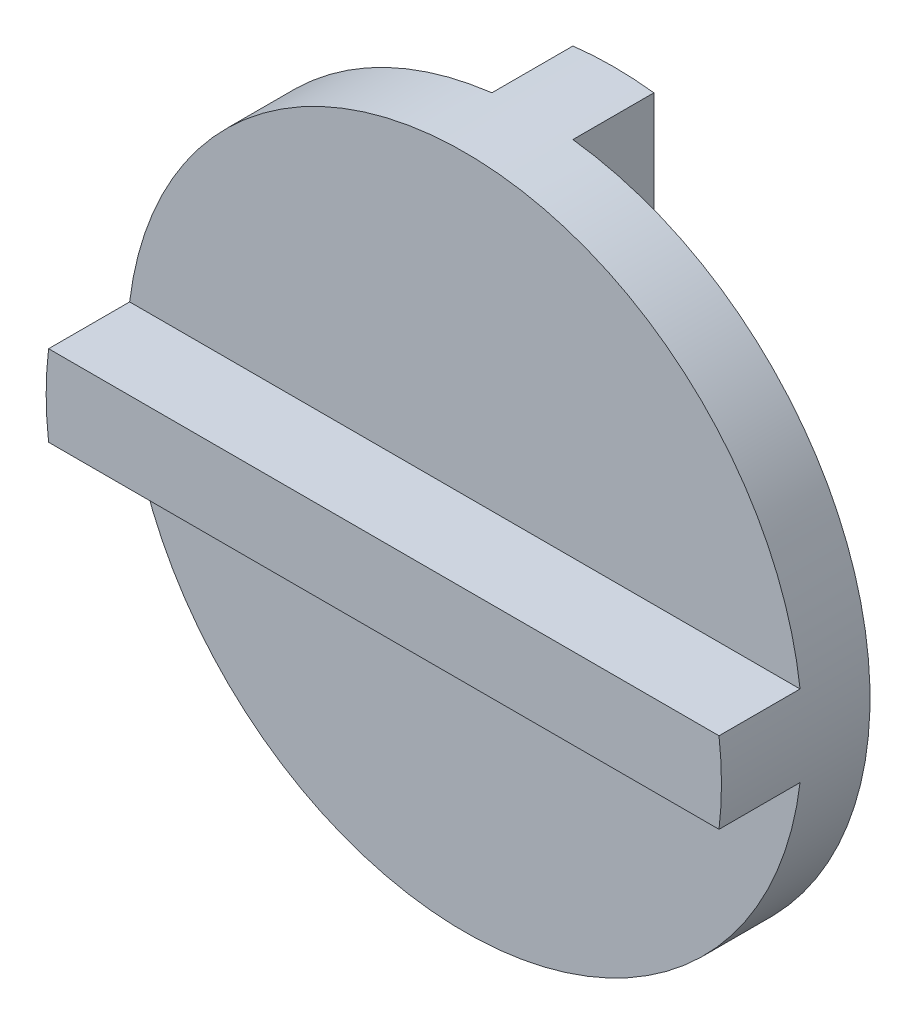
ISO-10303-21;
HEADER;
FILE_DESCRIPTION(('STEP AP214'),'2;1');
FILE_NAME('part.step','',(''),(''),'','','');
FILE_SCHEMA(('AUTOMOTIVE_DESIGN { 1 0 10303 214 1 1 1 1 }'));
ENDSEC;
DATA;
#1=APPLICATION_CONTEXT('core data for automotive mechanical design processes');
#2=APPLICATION_PROTOCOL_DEFINITION('international standard','automotive_design',2000,#1);
#3=PRODUCT_CONTEXT('',#1,'mechanical');
#4=PRODUCT('Part','Part','',(#3));
#5=PRODUCT_RELATED_PRODUCT_CATEGORY('part','',(#4));
#6=PRODUCT_DEFINITION_FORMATION('','',#4);
#7=PRODUCT_DEFINITION_CONTEXT('part definition',#1,'design');
#8=PRODUCT_DEFINITION('design','',#6,#7);
#9=PRODUCT_DEFINITION_SHAPE('','',#8);
#10=(LENGTH_UNIT() NAMED_UNIT(*) SI_UNIT(.MILLI.,.METRE.));
#11=(NAMED_UNIT(*) PLANE_ANGLE_UNIT() SI_UNIT($,.RADIAN.));
#12=(NAMED_UNIT(*) SI_UNIT($,.STERADIAN.) SOLID_ANGLE_UNIT());
#13=UNCERTAINTY_MEASURE_WITH_UNIT(LENGTH_MEASURE(1.E-05),#10,'distance_accuracy_value','');
#14=(GEOMETRIC_REPRESENTATION_CONTEXT(3) GLOBAL_UNCERTAINTY_ASSIGNED_CONTEXT((#13)) GLOBAL_UNIT_ASSIGNED_CONTEXT((#10,
#11,#12)) REPRESENTATION_CONTEXT('',''));
#15=CARTESIAN_POINT('',(0.,0.,0.));
#16=DIRECTION('',(0.,0.,1.));
#17=DIRECTION('',(1.,0.,0.));
#18=AXIS2_PLACEMENT_3D('',#15,#16,#17);
#19=CARTESIAN_POINT('',(0.,0.,-5.));
#20=DIRECTION('',(0.,0.,1.));
#21=DIRECTION('',(1.,0.,0.));
#22=AXIS2_PLACEMENT_3D('',#19,#20,#21);
#23=PLANE('',#22);
#24=DIRECTION('',(0.,1.,0.));
#25=VECTOR('',#24,1.);
#26=CARTESIAN_POINT('',(-6.,-49.6386945839634,-5.));
#27=LINE('',#26,#25);
#28=CARTESIAN_POINT('',(-6.,-49.6386945839634,-5.));
#29=VERTEX_POINT('',#28);
#30=CARTESIAN_POINT('',(-6.,49.6386945839634,-5.));
#31=VERTEX_POINT('',#30);
#32=EDGE_CURVE('E53',#29,#31,#27,.T.);
#33=ORIENTED_EDGE('',*,*,#32,.F.);
#34=CARTESIAN_POINT('',(0.,0.,-5.));
#35=DIRECTION('',(0.,0.,1.));
#36=DIRECTION('',(1.,0.,0.));
#37=AXIS2_PLACEMENT_3D('',#34,#35,#36);
#38=CIRCLE('',#37,50.);
#39=EDGE_CURVE('E60',#31,#29,#38,.T.);
#40=ORIENTED_EDGE('',*,*,#39,.F.);
#41=EDGE_LOOP('',(#33,#40));
#42=FACE_BOUND('',#41,.T.);
#43=ADVANCED_FACE('F39',(#42),#23,.F.);
#44=DIRECTION('',(0.,-1.,0.));
#45=VECTOR('',#44,1.);
#46=CARTESIAN_POINT('',(6.,-49.6386945839634,-5.));
#47=LINE('',#46,#45);
#48=CARTESIAN_POINT('',(6.,49.6386945839634,-5.));
#49=VERTEX_POINT('',#48);
#50=CARTESIAN_POINT('',(6.,-49.6386945839634,-5.));
#51=VERTEX_POINT('',#50);
#52=EDGE_CURVE('E280',#49,#51,#47,.T.);
#53=ORIENTED_EDGE('',*,*,#52,.F.);
#54=EDGE_CURVE('E43',#51,#49,#38,.T.);
#55=ORIENTED_EDGE('',*,*,#54,.F.);
#56=EDGE_LOOP('',(#53,#55));
#57=FACE_BOUND('',#56,.T.);
#58=ADVANCED_FACE('F180',(#57),#23,.F.);
#59=CARTESIAN_POINT('',(0.,0.,5.));
#60=DIRECTION('',(0.,0.,1.));
#61=DIRECTION('',(1.,0.,0.));
#62=AXIS2_PLACEMENT_3D('',#59,#60,#61);
#63=PLANE('',#62);
#64=DIRECTION('',(-1.,0.,0.));
#65=VECTOR('',#64,1.);
#66=CARTESIAN_POINT('',(49.6386945839634,6.,5.));
#67=LINE('',#66,#65);
#68=CARTESIAN_POINT('',(49.6386945839634,6.,5.));
#69=VERTEX_POINT('',#68);
#70=CARTESIAN_POINT('',(-49.6386945839634,6.,5.));
#71=VERTEX_POINT('',#70);
#72=EDGE_CURVE('E127',#69,#71,#67,.T.);
#73=ORIENTED_EDGE('',*,*,#72,.F.);
#74=CARTESIAN_POINT('',(0.,0.,5.));
#75=DIRECTION('',(0.,0.,1.));
#76=DIRECTION('',(1.,0.,0.));
#77=AXIS2_PLACEMENT_3D('',#74,#75,#76);
#78=CIRCLE('',#77,50.);
#79=EDGE_CURVE('E11',#69,#71,#78,.T.);
#80=ORIENTED_EDGE('',*,*,#79,.T.);
#81=EDGE_LOOP('',(#73,#80));
#82=FACE_BOUND('',#81,.T.);
#83=ADVANCED_FACE('F174',(#82),#63,.T.);
#84=CARTESIAN_POINT('',(0.,0.,5.));
#85=DIRECTION('',(0.,0.,-1.));
#86=DIRECTION('',(-1.,0.,0.));
#87=AXIS2_PLACEMENT_3D('',#84,#85,#86);
#88=CYLINDRICAL_SURFACE('',#87,50.);
#89=ORIENTED_EDGE('',*,*,#79,.F.);
#90=DIRECTION('',(0.,0.,-1.));
#91=VECTOR('',#90,1.);
#92=CARTESIAN_POINT('',(49.6386945839634,6.,17.));
#93=LINE('',#92,#91);
#94=CARTESIAN_POINT('',(49.6386945839634,6.,17.));
#95=VERTEX_POINT('',#94);
#96=EDGE_CURVE('E148',#95,#69,#93,.T.);
#97=ORIENTED_EDGE('',*,*,#96,.F.);
#98=CARTESIAN_POINT('',(0.,0.,17.));
#99=DIRECTION('',(0.,0.,1.));
#100=DIRECTION('',(1.,0.,0.));
#101=AXIS2_PLACEMENT_3D('',#98,#99,#100);
#102=CIRCLE('',#101,50.);
#103=CARTESIAN_POINT('',(49.6386945839634,-6.00000000000001,17.));
#104=VERTEX_POINT('',#103);
#105=EDGE_CURVE('E140',#104,#95,#102,.T.);
#106=ORIENTED_EDGE('',*,*,#105,.F.);
#107=DIRECTION('',(0.,0.,-1.));
#108=VECTOR('',#107,1.);
#109=CARTESIAN_POINT('',(49.6386945839634,-6.00000000000001,17.));
#110=LINE('',#109,#108);
#111=CARTESIAN_POINT('',(49.6386945839634,-6.00000000000001,5.));
#112=VERTEX_POINT('',#111);
#113=EDGE_CURVE('E149',#104,#112,#110,.T.);
#114=ORIENTED_EDGE('',*,*,#113,.T.);
#115=CARTESIAN_POINT('',(-49.6386945839634,-6.,5.));
#116=VERTEX_POINT('',#115);
#117=EDGE_CURVE('E48',#116,#112,#78,.T.);
#118=ORIENTED_EDGE('',*,*,#117,.F.);
#119=DIRECTION('',(0.,0.,-1.));
#120=VECTOR('',#119,1.);
#121=CARTESIAN_POINT('',(-49.6386945839634,-6.,17.));
#122=LINE('',#121,#120);
#123=CARTESIAN_POINT('',(-49.6386945839634,-6.,17.));
#124=VERTEX_POINT('',#123);
#125=EDGE_CURVE('E155',#124,#116,#122,.T.);
#126=ORIENTED_EDGE('',*,*,#125,.F.);
#127=CARTESIAN_POINT('',(0.,0.,17.));
#128=DIRECTION('',(0.,0.,1.));
#129=DIRECTION('',(1.,0.,0.));
#130=AXIS2_PLACEMENT_3D('',#127,#128,#129);
#131=CIRCLE('',#130,50.);
#132=CARTESIAN_POINT('',(-49.6386945839634,6.,17.));
#133=VERTEX_POINT('',#132);
#134=EDGE_CURVE('E135',#133,#124,#131,.T.);
#135=ORIENTED_EDGE('',*,*,#134,.F.);
#136=DIRECTION('',(0.,0.,-1.));
#137=VECTOR('',#136,1.);
#138=CARTESIAN_POINT('',(-49.6386945839634,6.,17.));
#139=LINE('',#138,#137);
#140=EDGE_CURVE('E136',#133,#71,#139,.T.);
#141=ORIENTED_EDGE('',*,*,#140,.T.);
#142=EDGE_LOOP('',(#89,#97,#106,#114,#118,#126,#135,#141));
#143=FACE_BOUND('',#142,.T.);
#144=ORIENTED_EDGE('',*,*,#54,.T.);
#145=DIRECTION('',(0.,0.,1.));
#146=VECTOR('',#145,1.);
#147=CARTESIAN_POINT('',(6.,49.6386945839634,-17.));
#148=LINE('',#147,#146);
#149=CARTESIAN_POINT('',(6.,49.6386945839634,-17.));
#150=VERTEX_POINT('',#149);
#151=EDGE_CURVE('E106',#150,#49,#148,.T.);
#152=ORIENTED_EDGE('',*,*,#151,.F.);
#153=CARTESIAN_POINT('',(0.,0.,-17.));
#154=DIRECTION('',(0.,0.,-1.));
#155=DIRECTION('',(-1.,0.,0.));
#156=AXIS2_PLACEMENT_3D('',#153,#154,#155);
#157=CIRCLE('',#156,50.);
#158=CARTESIAN_POINT('',(-6.,49.6386945839634,-17.));
#159=VERTEX_POINT('',#158);
#160=EDGE_CURVE('E115',#159,#150,#157,.T.);
#161=ORIENTED_EDGE('',*,*,#160,.F.);
#162=DIRECTION('',(0.,0.,1.));
#163=VECTOR('',#162,1.);
#164=CARTESIAN_POINT('',(-6.,49.6386945839634,-17.));
#165=LINE('',#164,#163);
#166=EDGE_CURVE('E277',#159,#31,#165,.T.);
#167=ORIENTED_EDGE('',*,*,#166,.T.);
#168=ORIENTED_EDGE('',*,*,#39,.T.);
#169=DIRECTION('',(0.,0.,1.));
#170=VECTOR('',#169,1.);
#171=CARTESIAN_POINT('',(-6.,-49.6386945839634,-17.));
#172=LINE('',#171,#170);
#173=CARTESIAN_POINT('',(-6.,-49.6386945839634,-17.));
#174=VERTEX_POINT('',#173);
#175=EDGE_CURVE('E126',#174,#29,#172,.T.);
#176=ORIENTED_EDGE('',*,*,#175,.F.);
#177=CARTESIAN_POINT('',(0.,0.,-17.));
#178=DIRECTION('',(0.,0.,-1.));
#179=DIRECTION('',(-1.,0.,0.));
#180=AXIS2_PLACEMENT_3D('',#177,#178,#179);
#181=CIRCLE('',#180,50.);
#182=CARTESIAN_POINT('',(6.,-49.6386945839634,-17.));
#183=VERTEX_POINT('',#182);
#184=EDGE_CURVE('E112',#183,#174,#181,.T.);
#185=ORIENTED_EDGE('',*,*,#184,.F.);
#186=DIRECTION('',(0.,0.,1.));
#187=VECTOR('',#186,1.);
#188=CARTESIAN_POINT('',(6.,-49.6386945839634,-17.));
#189=LINE('',#188,#187);
#190=EDGE_CURVE('E107',#183,#51,#189,.T.);
#191=ORIENTED_EDGE('',*,*,#190,.T.);
#192=EDGE_LOOP('',(#144,#152,#161,#167,#168,#176,#185,#191));
#193=FACE_BOUND('',#192,.T.);
#194=ADVANCED_FACE('F41',(#143,#193),#88,.T.);
#195=DIRECTION('',(1.,0.,0.));
#196=VECTOR('',#195,1.);
#197=CARTESIAN_POINT('',(49.6386945839634,-6.,5.));
#198=LINE('',#197,#196);
#199=EDGE_CURVE('E123',#116,#112,#198,.T.);
#200=ORIENTED_EDGE('',*,*,#199,.F.);
#201=ORIENTED_EDGE('',*,*,#117,.T.);
#202=EDGE_LOOP('',(#200,#201));
#203=FACE_BOUND('',#202,.T.);
#204=ADVANCED_FACE('F159',(#203),#63,.T.);
#205=CARTESIAN_POINT('',(49.6386945839634,-6.,17.));
#206=DIRECTION('',(0.,1.,0.));
#207=DIRECTION('',(0.,0.,1.));
#208=AXIS2_PLACEMENT_3D('',#205,#206,#207);
#209=PLANE('',#208);
#210=ORIENTED_EDGE('',*,*,#199,.T.);
#211=ORIENTED_EDGE('',*,*,#113,.F.);
#212=DIRECTION('',(1.,0.,0.));
#213=VECTOR('',#212,1.);
#214=CARTESIAN_POINT('',(49.6386945839634,-6.,17.));
#215=LINE('',#214,#213);
#216=EDGE_CURVE('E134',#124,#104,#215,.T.);
#217=ORIENTED_EDGE('',*,*,#216,.F.);
#218=ORIENTED_EDGE('',*,*,#125,.T.);
#219=EDGE_LOOP('',(#210,#211,#217,#218));
#220=FACE_BOUND('',#219,.T.);
#221=ADVANCED_FACE('F162',(#220),#209,.F.);
#222=CARTESIAN_POINT('',(49.6386945839634,6.,17.));
#223=DIRECTION('',(0.,-1.,0.));
#224=DIRECTION('',(0.,0.,-1.));
#225=AXIS2_PLACEMENT_3D('',#222,#223,#224);
#226=PLANE('',#225);
#227=ORIENTED_EDGE('',*,*,#72,.T.);
#228=ORIENTED_EDGE('',*,*,#140,.F.);
#229=DIRECTION('',(-1.,0.,0.));
#230=VECTOR('',#229,1.);
#231=CARTESIAN_POINT('',(49.6386945839634,6.,17.));
#232=LINE('',#231,#230);
#233=EDGE_CURVE('E139',#95,#133,#232,.T.);
#234=ORIENTED_EDGE('',*,*,#233,.F.);
#235=ORIENTED_EDGE('',*,*,#96,.T.);
#236=EDGE_LOOP('',(#227,#228,#234,#235));
#237=FACE_BOUND('',#236,.T.);
#238=ADVANCED_FACE('F172',(#237),#226,.F.);
#239=CARTESIAN_POINT('',(0.,0.,17.));
#240=DIRECTION('',(0.,0.,1.));
#241=DIRECTION('',(1.,0.,0.));
#242=AXIS2_PLACEMENT_3D('',#239,#240,#241);
#243=PLANE('',#242);
#244=ORIENTED_EDGE('',*,*,#134,.T.);
#245=ORIENTED_EDGE('',*,*,#216,.T.);
#246=ORIENTED_EDGE('',*,*,#105,.T.);
#247=ORIENTED_EDGE('',*,*,#233,.T.);
#248=EDGE_LOOP('',(#244,#245,#246,#247));
#249=FACE_BOUND('',#248,.T.);
#250=ADVANCED_FACE('F166',(#249),#243,.T.);
#251=CARTESIAN_POINT('',(6.,-49.6386945839634,-17.));
#252=DIRECTION('',(-1.,0.,0.));
#253=DIRECTION('',(0.,0.,1.));
#254=AXIS2_PLACEMENT_3D('',#251,#252,#253);
#255=PLANE('',#254);
#256=ORIENTED_EDGE('',*,*,#52,.T.);
#257=ORIENTED_EDGE('',*,*,#190,.F.);
#258=DIRECTION('',(0.,-1.,0.));
#259=VECTOR('',#258,1.);
#260=CARTESIAN_POINT('',(6.,-49.6386945839634,-17.));
#261=LINE('',#260,#259);
#262=EDGE_CURVE('E101',#150,#183,#261,.T.);
#263=ORIENTED_EDGE('',*,*,#262,.F.);
#264=ORIENTED_EDGE('',*,*,#151,.T.);
#265=EDGE_LOOP('',(#256,#257,#263,#264));
#266=FACE_BOUND('',#265,.T.);
#267=ADVANCED_FACE('F102',(#266),#255,.F.);
#268=CARTESIAN_POINT('',(-6.,-49.6386945839634,-17.));
#269=DIRECTION('',(1.,0.,0.));
#270=DIRECTION('',(0.,0.,-1.));
#271=AXIS2_PLACEMENT_3D('',#268,#269,#270);
#272=PLANE('',#271);
#273=ORIENTED_EDGE('',*,*,#32,.T.);
#274=ORIENTED_EDGE('',*,*,#166,.F.);
#275=DIRECTION('',(0.,1.,0.));
#276=VECTOR('',#275,1.);
#277=CARTESIAN_POINT('',(-6.,-49.6386945839634,-17.));
#278=LINE('',#277,#276);
#279=EDGE_CURVE('E120',#174,#159,#278,.T.);
#280=ORIENTED_EDGE('',*,*,#279,.F.);
#281=ORIENTED_EDGE('',*,*,#175,.T.);
#282=EDGE_LOOP('',(#273,#274,#280,#281));
#283=FACE_BOUND('',#282,.T.);
#284=ADVANCED_FACE('F209',(#283),#272,.F.);
#285=CARTESIAN_POINT('',(0.,0.,-17.));
#286=DIRECTION('',(0.,0.,-1.));
#287=DIRECTION('',(-1.,0.,0.));
#288=AXIS2_PLACEMENT_3D('',#285,#286,#287);
#289=PLANE('',#288);
#290=ORIENTED_EDGE('',*,*,#160,.T.);
#291=ORIENTED_EDGE('',*,*,#262,.T.);
#292=ORIENTED_EDGE('',*,*,#184,.T.);
#293=ORIENTED_EDGE('',*,*,#279,.T.);
#294=EDGE_LOOP('',(#290,#291,#292,#293));
#295=FACE_BOUND('',#294,.T.);
#296=ADVANCED_FACE('F113',(#295),#289,.T.);
#297=CLOSED_SHELL('',(#43,#58,#83,#194,#204,#221,#238,#250,#267,#284,#296));
#298=MANIFOLD_SOLID_BREP('B2',#297);
#299=ADVANCED_BREP_SHAPE_REPRESENTATION('',(#18,#298),#14);
#300=SHAPE_DEFINITION_REPRESENTATION(#9,#299);
ENDSEC;
END-ISO-10303-21;
